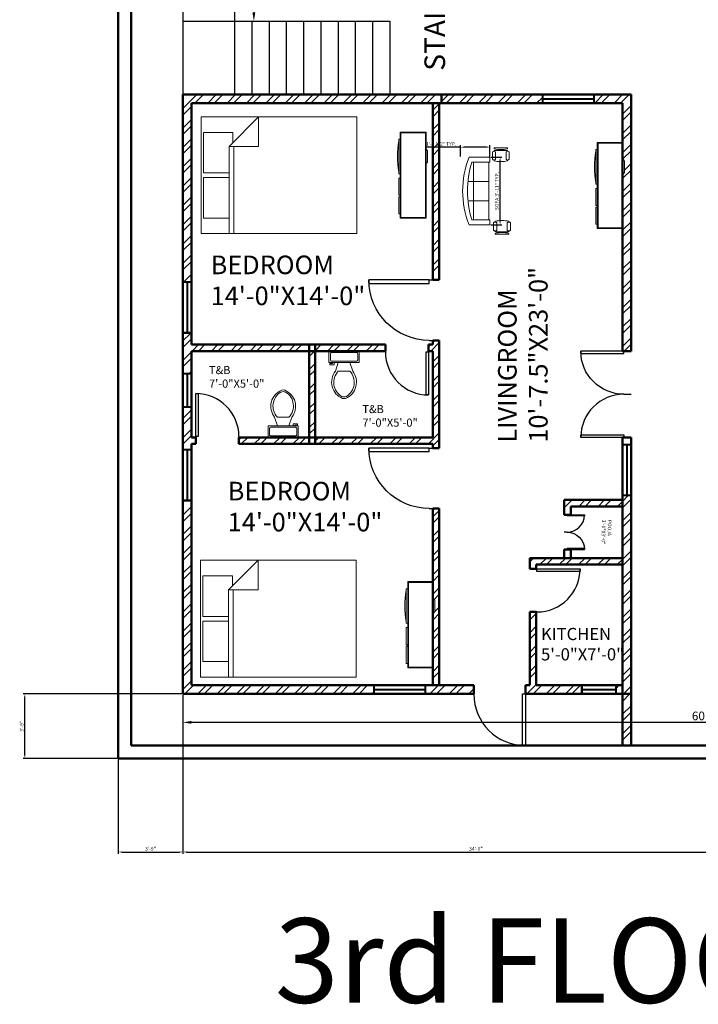
# Model space of a CAD drawing. Units: inches. Extents: x -12550 to 6516, y 1273 to 18700.
# Tile 12 of 19: x 4339 to 4811, y 1273 to 1958. Entities that reach past the tile are written whole.
import ezdxf

# ---------------------------------------------------------------- set-up
doc = ezdxf.new("R2010")
doc.units = ezdxf.units.IN
for name, color, linetype, lineweight in [('A-ANNO-DIMS', 2, 'Continuous', 18), ('A-ANNO-TEXT', 7, 'Continuous', 25), ('A-AREA-IDEN', 1, 'Continuous', 18), ('A-DOOR', 5, 'Continuous', 25), ('A-FLOR-STRS', 6, 'Continuous', 25), ('A-FURN', 8, 'Continuous', 18), ('A-GLAZ', 3, 'Continuous', 25), ('A-WALL', 7, 'Continuous', 50), ('A-WALL-PATT', 8, 'Continuous', 13)]:
    doc.layers.add(name, color=color, linetype=linetype, lineweight=lineweight)
doc.styles.get("Standard").update_dxf_attribs({"font": 'arial.ttf'})
doc.dimstyles.new('ISO-25', dxfattribs={"dimtxt": 2.5, "dimasz": 2.5, "dimexe": 1.25, "dimexo": 0.625, "dimtad": 1, "dimlunit": 4, "dimtxsty": 'Standard', "dimcen": 2.5, "dimadec": 0, "dimazin": 0, "dimtfac": 1, "dimtmove": 0, "dimatfit": 3, "dimfxl": 1, "dimarcsym": 0})
pattern_1 = [(45, (2434.941, 0), (-6.735192, 6.735192), []), (45, (2439.432, 0), (-6.735192, 6.735192), [])]

# ---------------------------------------------------------------- blocks, each defined once
blk = doc.blocks.new('*U2')
for p, q in [((0, 0), (0, -5)), ((30, 0), (30, -5))]:
    blk.add_line(p, q)
blk.add_lwpolyline([(0, 0), (0, 30), (1.75, 30), (1.75, 0)], close=True)
blk.add_arc((0, 0), 30, 0, 90)
blk = doc.blocks.new('Bed - Queen')
for p, q in [((0, -80.00003), (0, 0)), ((0, 0), (59.99999, 0)), ((59.99999, 0), (59.99999, -80.00003)), ((7.99999, -1.2), (28.79998, -1.2)), ((7.99999, -14.4), (7.99999, -1.2)), ((28.79998, -1.2), (28.79998, -14.4)), ((31.19999, -1.2), (51.99999, -1.2)), ((31.19999, -14.4), (31.19999, -1.2)), ((51.99999, -1.2), (51.99999, -16.4)), ((0, -14.4), (44.8, -14.4)), ((59.99999, -29.6), (44.8, -14.4)), ((44.8, -14.4), (44.8, -29.6)), ((44.8, -16.8), (0, -16.8)), ((51.99999, -16.4), (46.79936, -16.4)), ((44.8, -29.6), (59.99999, -29.6)), ((59.99999, -80.00003), (0, -80.00003))]:
    blk.add_line(p, q)
blk = doc.blocks.new('Toilet - top')
for p, q in [((9.5, -6), (9.5, -2)), ((-10, -8.5), (-8, -8.5)), ((-10, -9.5), (-10, -8.5)), ((-7, -9.5), (-10, -9.5)), ((-8, -8.5), (-8, -8)), ((-7, -8), (-7, -9.5)), ((-4, -8), (-6, -14)), ((4, -8), (6, -14)), ((4, -14), (-4, -14))]:
    blk.add_line(p, q)
blk.add_lwpolyline([(10.5, -8), (10.5, 0), (-10.5, 0), (-10.5, -8)], close=True)
for points in [[(-9.5, -2), (-9.5, -6)], [(8.5, -1), (-8.5, -1)], [(-8.5, -7), (8.5, -7)]]:
    blk.add_lwpolyline(points)
for centre, radius, start, end in [((-8.62, -1.88), 0.884, 81.8699, 188.1301), ((-8.62, -6.12), 0.884, 171.8699, 278.1301), ((8.62, -1.88), 0.884, 351.8699, 98.1301), ((8.62, -6.12), 0.884, 261.8699, 8.1301), ((3.52, -21.58), 12.17, 141.46911, 247.97143), ((4.2, -21.82), 11.33, 136.36773, 238.94682), ((-3.52, -21.58), 12.17, 292.02843, 38.53071), ((-4.2, -21.82), 11.33, 301.05301, 43.63209), ((0, -27.88), 4, 245.73182, 294.26817), ((0, -29), 4, 254.86053, 285.13947)]:
    blk.add_arc(centre, radius, start, end)
blk = doc.blocks.new('Entertainment Center')
for p, q in [((-4, 0), (-5, -1)), ((4, 0), (-4, 0)), ((5, -1), (4, 0)), ((-17, -19), (-17, -1)), ((-17, -1), (43, -1)), ((-16.5, -18.5), (-16.5, -1.5)), ((-16.5, -1.5), (42.5, -1.5)), ((42.5, -1.5), (42.5, -18.5)), ((43, -1), (43, -19)), ((43, -19), (-17, -19)), ((42.5, -18.5), (-16.5, -18.5)), ((-12, -20), (-12, -19)), ((12, -20), (-12, -20)), ((12, -19), (12, -20)), ((15, -20), (15, -19)), ((27, -20), (15, -20)), ((27, -19), (27, -20)), ((28, -20), (28, -19)), ((40, -20), (28, -20)), ((40, -19), (40, -20))]:
    blk.add_line(p, q)
blk.add_arc((0, 40), 61, 259.6111, 280.3889)
blk = doc.blocks.new('Sofa - Roundback 7 ft.')
for p, q in [((-36.000027, -34), (-36.000027, -11.4696)), ((-12.00002, -32.4421), (-12.00003, -6.5971)), ((11.99997, -32.4421), (11.99998, -6.5971)), ((35.99998, -34), (35.99998, -11.4696)), ((-35.999844, -13.3819), (35.9998, -13.3819)), ((-36.000027, -32.4421), (35.99998, -32.4421))]:
    blk.add_line(p, q)
for points in [[(-36.000027, -34), (-42.000027, -34), (-42.000027, -8)], [(41.99998, -8), (41.99998, -34), (35.99998, -34)]]:
    blk.add_lwpolyline(points)
for centre, radius, start, end in [((0, -114.25), 114.25, 68.43141, 111.5686), ((-0.00001, -127.1968), 121.1968, 72.72033, 107.2797)]:
    blk.add_arc(centre, radius, start, end)
blk = doc.blocks.new('Chair - Desk')
for p, q in [((-8.5, 0), (-8.5, -1)), ((-8.5, 0), (8.5, 0)), ((8.5, 0), (8.5, -1)), ((-10.5, -5), (-10.5, -14)), ((-8.5, -3), (-8.5, -4)), ((-8.5, -3), (8.5, -3)), ((-6.5, -14), (-6.5, -5)), ((-2, -3), (-2, -1.9355)), ((2, -1.9576), (2, -3)), ((6.5, -5), (6.5, -14)), ((8.5, -3), (8.5, -4)), ((10.5, -14), (10.5, -5)), ((-8.5, -15), (-8.5, -16)), ((8.5, -15), (8.5, -16))]:
    blk.add_line(p, q)
for centre, radius, start, end in [((-8.5, -6.5), 2.5, 36.8699, 143.1301), ((0, 34.625), 36.625, 256.5803, 283.4197), ((8.5, -6.5), 2.5, 36.8699, 143.1301), ((-8.5, -12.5), 2.5, 216.8699, 323.1301), ((0, 19.625), 36.625, 256.5803, 283.4197), ((8.5, -12.5), 2.5, 216.8699, 323.1301)]:
    blk.add_arc(centre, radius, start, end)
blk = doc.blocks.new('*D48')
at = {"layer": 'A-ANNO-DIMS', "color": 0, "lineweight": -2, "transparency": 16777216}
for p, q in [((4489.26, 2008.25), (4503.3, 2008.25)), ((4502.05, 2002.25), (4502.05, 1963.25)), ((4489.26, 1957.25), (4503.3, 1957.25))]:
    blk.add_line(p, q, dxfattribs=at)
at = {"layer": 'A-ANNO-DIMS', "color": 0, "transparency": 16777216}
for points in [[(4501.05, 2002.25), (4503.05, 2002.25), (4502.05, 2008.25)], [(4501.05, 1963.25), (4503.05, 1963.25), (4502.05, 1957.25)]]:
    blk.add_solid(points, dxfattribs=at)
at = {"layer": 'Defpoints', "color": 0, "transparency": 16777216}
for p in [(4488.63, 2008.25), (4488.63, 1957.25), (4502.05, 1957.25)]:
    blk.add_point(p, dxfattribs=at)
at = {"layer": 'A-ANNO-DIMS', "color": 0, "transparency": 16777216, "insert": (4498.36, 1982.75), "char_height": 6, "attachment_point": 5, "rotation": 90}
blk.add_mtext('4\'-3"', dxfattribs=at)
blk = doc.blocks.new('*D43')
at = {"layer": 'A-ANNO-DIMS', "color": 0, "lineweight": -2, "transparency": 16777216}
for p, q in [((4452.63, 1488.62), (4452.63, 1468.21)), ((5172.63, 1488.62), (5172.63, 1468.21)), ((5166.63, 1469.46), (4458.63, 1469.46))]:
    blk.add_line(p, q, dxfattribs=at)
at = {"layer": 'A-ANNO-DIMS', "color": 0, "transparency": 16777216}
for points in [[(4458.63, 1470.46), (4458.63, 1468.46), (4452.63, 1469.46)], [(5166.63, 1470.46), (5166.63, 1468.46), (5172.63, 1469.46)]]:
    blk.add_solid(points, dxfattribs=at)
at = {"layer": 'Defpoints', "color": 0, "transparency": 16777216}
for p in [(4452.63, 1489.25), (5172.63, 1489.25), (4452.63, 1469.46)]:
    blk.add_point(p, dxfattribs=at)
at = {"layer": 'A-ANNO-DIMS', "color": 0, "transparency": 16777216, "insert": (4812.63, 1473.15), "char_height": 6, "attachment_point": 5}
blk.add_mtext("60'", dxfattribs=at)
blk = doc.blocks.new('WIN-3FT')
for p, q in [((0, 0), (0, 6)), ((0, 6), (36.02, 6)), ((36.02, 0), (0, 0)), ((0.5, 0), (0.5, 6)), ((35.52, 3.2), (0.5, 3.2)), ((35.52, 2.8), (0.5, 2.8)), ((35.52, 6), (35.52, 0)), ((36.02, 6), (36.02, 0))]:
    blk.add_line(p, q)
blk = doc.blocks.new('WIN-2FT')
for p, q in [((0, 0), (0, 24.02)), ((0, 24.02), (6, 24.02)), ((0, 23.52), (6, 23.52)), ((2.8, 0.5), (2.8, 23.52)), ((3.2, 0.5), (3.2, 23.52)), ((6, 24.02), (6, 0)), ((6, 0.5), (0, 0.5)), ((6, 0), (0, 0))]:
    blk.add_line(p, q)
blk = doc.blocks.new('*D75')
at = {"layer": 'A-ANNO-DIMS', "color": 0, "lineweight": -2, "transparency": 16777216}
for p, q in [((4667.04, 1862.64), (4674.71, 1862.64)), ((4673.46, 1818.14), (4673.46, 1860.14)), ((4667.04, 1815.64), (4674.71, 1815.64))]:
    blk.add_line(p, q, dxfattribs=at)
at = {"layer": 'A-ANNO-DIMS', "color": 0, "transparency": 16777216}
for points in [[(4673.05, 1860.14), (4673.88, 1860.14), (4673.46, 1862.64)], [(4673.05, 1818.14), (4673.88, 1818.14), (4673.46, 1815.64)]]:
    blk.add_solid(points, dxfattribs=at)
at = {"layer": 'Defpoints', "color": 0, "transparency": 16777216}
for p in [(4666.41, 1862.64), (4673.46, 1862.64), (4666.41, 1815.64)]:
    blk.add_point(p, dxfattribs=at)
at = {"layer": 'A-ANNO-DIMS', "color": 0, "transparency": 16777216, "insert": (4671.54, 1839.14), "char_height": 2.5, "attachment_point": 5, "rotation": 90}
blk.add_mtext('SOFA 3\'-11" TYP.', dxfattribs=at)
blk = doc.blocks.new('*D76')
at = {"layer": 'A-ANNO-DIMS', "color": 0, "lineweight": -2, "transparency": 16777216}
for p, q in [((4645.9, 1863.26), (4645.9, 1870.94)), ((4666.41, 1863.26), (4666.41, 1870.94)), ((4645.9, 1869.69), (4621.32, 1869.69)), ((4663.91, 1869.69), (4648.4, 1869.69))]:
    blk.add_line(p, q, dxfattribs=at)
at = {"layer": 'A-ANNO-DIMS', "color": 0, "transparency": 16777216}
for points in [[(4648.4, 1870.1), (4648.4, 1869.27), (4645.9, 1869.69)], [(4663.91, 1870.1), (4663.91, 1869.27), (4666.41, 1869.69)]]:
    blk.add_solid(points, dxfattribs=at)
at = {"layer": 'Defpoints', "color": 0, "transparency": 16777216}
for p in [(4645.9, 1869.69), (4645.9, 1862.64), (4666.41, 1862.64)]:
    blk.add_point(p, dxfattribs=at)
at = {"layer": 'A-ANNO-DIMS', "color": 0, "transparency": 16777216, "insert": (4632.36, 1871.61), "char_height": 2.5, "attachment_point": 5}
blk.add_mtext('1\'-8 1/2" TYP.', dxfattribs=at)
blk = doc.blocks.new('*D114')
at = {"layer": 'A-ANNO-DIMS', "color": 0, "lineweight": -2, "transparency": 16777216}
for p, q in [((4452.63, 1488.62), (4452.63, 1378)), ((4407.63, 1443.62), (4407.63, 1378)), ((4410.13, 1379.25), (4450.13, 1379.25))]:
    blk.add_line(p, q, dxfattribs=at)
at = {"layer": 'A-ANNO-DIMS', "color": 0, "transparency": 16777216}
for points in [[(4410.13, 1379.66), (4410.13, 1378.83), (4407.63, 1379.25)], [(4450.13, 1379.66), (4450.13, 1378.83), (4452.63, 1379.25)]]:
    blk.add_solid(points, dxfattribs=at)
at = {"layer": 'Defpoints', "color": 0, "transparency": 16777216}
for p in [(4452.63, 1489.25), (4407.63, 1444.25), (4452.63, 1379.25)]:
    blk.add_point(p, dxfattribs=at)
at = {"layer": 'A-ANNO-DIMS', "color": 0, "transparency": 16777216, "insert": (4430.13, 1381.15), "char_height": 2.5, "attachment_point": 5}
blk.add_mtext('3\'-9"', dxfattribs=at)
blk = doc.blocks.new('*D115')
at = {"layer": 'A-ANNO-DIMS', "color": 0, "lineweight": -2, "transparency": 16777216}
for p, q in [((4452.63, 1488.62), (4452.63, 1378)), ((4860.63, 1488.62), (4860.63, 1378)), ((4455.13, 1379.25), (4858.13, 1379.25))]:
    blk.add_line(p, q, dxfattribs=at)
at = {"layer": 'A-ANNO-DIMS', "color": 0, "transparency": 16777216}
for points in [[(4455.13, 1379.66), (4455.13, 1378.83), (4452.63, 1379.25)], [(4858.13, 1379.66), (4858.13, 1378.83), (4860.63, 1379.25)]]:
    blk.add_solid(points, dxfattribs=at)
at = {"layer": 'Defpoints', "color": 0, "transparency": 16777216}
for p in [(4452.63, 1489.25), (4860.63, 1489.25), (4860.63, 1379.25)]:
    blk.add_point(p, dxfattribs=at)
at = {"layer": 'A-ANNO-DIMS', "color": 0, "transparency": 16777216, "insert": (4656.63, 1381.15), "char_height": 2.5, "attachment_point": 5}
blk.add_mtext('34\'-0"', dxfattribs=at)
blk = doc.blocks.new('*D119')
at = {"layer": 'A-ANNO-DIMS', "color": 0, "lineweight": -2, "transparency": 16777216}
for p, q in [((4452.01, 1489.25), (4341.38, 1489.25)), ((4342.63, 1446.75), (4342.63, 1486.75)), ((4407.01, 1444.25), (4341.38, 1444.25))]:
    blk.add_line(p, q, dxfattribs=at)
at = {"layer": 'A-ANNO-DIMS', "color": 0, "transparency": 16777216}
for points in [[(4342.21, 1486.75), (4343.05, 1486.75), (4342.63, 1489.25)], [(4342.21, 1446.75), (4343.05, 1446.75), (4342.63, 1444.25)]]:
    blk.add_solid(points, dxfattribs=at)
at = {"layer": 'Defpoints', "color": 0, "transparency": 16777216}
for p in [(4342.63, 1489.25), (4452.63, 1489.25), (4407.63, 1444.25)]:
    blk.add_point(p, dxfattribs=at)
at = {"layer": 'A-ANNO-DIMS', "color": 0, "transparency": 16777216, "insert": (4340.73, 1466.75), "char_height": 2.5, "attachment_point": 5, "rotation": 90}
blk.add_mtext('3\'-9"', dxfattribs=at)

msp = doc.modelspace()

# ---------------------------------------------------------------- hatches: boundary and pattern name
at = {"layer": 'A-WALL-PATT'}
h = msp.add_hatch(dxfattribs=at)
h.set_pattern_fill('ANSI32', color=256)
h.set_pattern_definition(pattern_1)
h.paths.add_polyline_path([(4458.63, 1900.247), (4632.63, 1900.247), (4632.63, 1906.247), (4452.63, 1906.247), (4452.63, 1776.138), (4458.63, 1776.138)])
h = msp.add_hatch(dxfattribs=at)
h.set_pattern_fill('ANSI32', color=256)
h.set_pattern_definition(pattern_1)
h.paths.add_polyline_path([(4702.882, 1906.247), (4632.63, 1906.247), (4632.63, 1900.247), (4702.882, 1900.247)])
h = msp.add_hatch(dxfattribs=at)
h.set_pattern_fill('ANSI32', color=256)
h.set_pattern_definition(pattern_1)
h.paths.add_polyline_path([(4764.63, 1906.247), (4738.899, 1906.247), (4738.899, 1900.247), (4758.63, 1900.247), (4758.63, 1872.972), (4759.13, 1872.972), (4759.13, 1860.972), (4760.13, 1859.972), (4760.13, 1851.972), (4759.13, 1850.972), (4759.13, 1812.972), (4758.63, 1727.747), (4759.63, 1727.747), (4764.63, 1727.747)])
h = msp.add_hatch(dxfattribs=at)
h.set_pattern_fill('ANSI32', color=256)
h.set_pattern_definition(pattern_1)
h.paths.add_polyline_path([(4631.13, 1900.247), (4626.63, 1900.247), (4626.63, 1777.247), (4631.13, 1777.247)], flags=17)
h = msp.add_hatch(dxfattribs=at)
h.set_pattern_fill('ANSI32', color=256)
h.set_pattern_definition(pattern_1)
h.paths.add_polyline_path([(4540.63, 1732.247), (4458.63, 1732.247), (4458.63, 1740.121), (4452.63, 1740.121), (4452.63, 1712.466), (4458.63, 1712.466), (4458.63, 1727.747), (4540.63, 1727.747)])
h = msp.add_hatch(dxfattribs=at)
h.set_pattern_fill('ANSI32', color=256)
h.set_pattern_definition(pattern_1)
h.paths.add_polyline_path([(4631.13, 1735.247), (4626.63, 1735.247), (4626.63, 1732.247), (4623.63, 1732.247), (4623.63, 1727.747), (4626.63, 1727.747), (4626.63, 1667.747), (4544.63, 1667.747), (4544.63, 1663.247), (4626.63, 1663.247), (4626.63, 1660.247), (4631.13, 1660.247)])
h = msp.add_hatch(dxfattribs=at)
h.set_pattern_fill('ANSI32', color=256)
h.set_pattern_definition(pattern_1)
h.paths.add_polyline_path([(4544.63, 1727.747), (4540.63, 1727.747), (4540.63, 1667.747), (4544.63, 1667.747)])
h = msp.add_hatch(dxfattribs=at)
h.set_pattern_fill('ANSI32', color=256)
h.set_pattern_definition(pattern_1)
h.paths.add_polyline_path([(4593.63, 1732.247), (4544.63, 1732.247), (4544.63, 1727.747), (4593.63, 1727.747)], flags=17)
h = msp.add_hatch(dxfattribs=at)
h.set_pattern_fill('ANSI32', color=256)
h.set_pattern_definition(pattern_1)
h.paths.add_polyline_path([(4458.63, 1688.449), (4452.63, 1688.449), (4452.63, 1659.453), (4458.63, 1659.453), (4458.63, 1663.247), (4461.63, 1663.247), (4461.63, 1667.747), (4458.63, 1667.747)])
h = msp.add_hatch(dxfattribs=at)
h.set_pattern_fill('ANSI32', color=256)
h.set_pattern_definition(pattern_1)
h.paths.add_polyline_path([(4540.63, 1667.747), (4491.63, 1667.747), (4491.63, 1663.247), (4540.63, 1663.247)])
h = msp.add_hatch(dxfattribs=at)
h.set_pattern_fill('ANSI32', color=256)
h.set_pattern_definition(pattern_1)
h.paths.add_polyline_path([(4758.63, 1624.247), (4718.13, 1624.247), (4718.13, 1613.747), (4720.13, 1613.747), (4722.63, 1613.747), (4722.63, 1619.747), (4758.63, 1619.747)])
h = msp.add_hatch(dxfattribs=at)
h.set_pattern_fill('ANSI32', color=256)
h.set_pattern_definition(pattern_1)
h.paths.add_polyline_path([(4764.63, 1627.032), (4758.63, 1627.032), (4758.63, 1495.247), (4754.235, 1495.247), (4754.235, 1489.247), (4764.63, 1489.247)])
h = msp.add_hatch(dxfattribs=at)
h.set_pattern_fill('ANSI32', color=256)
h.set_pattern_definition(pattern_1)
h.paths.add_polyline_path([(4458.63, 1623.435), (4452.63, 1623.435), (4452.63, 1489.247), (4585.581, 1489.247), (4585.581, 1495.247), (4458.63, 1495.247)])
h = msp.add_hatch(dxfattribs=at)
h.set_pattern_fill('ANSI32', color=256)
h.set_pattern_definition(pattern_1)
h.paths.add_polyline_path([(4631.13, 1618.247), (4626.63, 1618.247), (4626.63, 1567.365), (4627.13, 1567.365), (4627.13, 1555.365), (4628.13, 1554.365), (4628.13, 1546.365), (4627.13, 1545.365), (4627.13, 1507.365), (4626.63, 1495.247), (4631.13, 1495.247)])
h = msp.add_hatch(dxfattribs=at)
h.set_pattern_fill('ANSI32', color=256)
h.set_pattern_definition(pattern_1)
h.paths.add_polyline_path([(4758.63, 1583.747), (4694.13, 1583.747), (4694.13, 1576.247), (4698.63, 1576.247), (4698.63, 1579.247), (4758.63, 1579.247)])
h = msp.add_hatch(dxfattribs=at)
h.set_pattern_fill('ANSI32', color=256)
h.set_pattern_definition(pattern_1)
h.paths.add_polyline_path([(4730.218, 1495.247), (4698.63, 1495.247), (4698.63, 1546.247), (4694.13, 1546.247), (4694.13, 1495.247), (4691.13, 1495.247), (4691.13, 1489.247), (4730.218, 1489.247)])
h = msp.add_hatch(dxfattribs=at)
h.set_pattern_fill('ANSI32', color=256)
h.set_pattern_definition(pattern_1)
h.paths.add_polyline_path([(4655.13, 1495.247), (4621.598, 1495.247), (4621.598, 1489.247), (4655.13, 1489.247)])
h = msp.add_hatch(dxfattribs=at)
h.set_pattern_fill('ANSI32', color=256)
h.set_pattern_definition(pattern_1)
h.paths.add_polyline_path([(4764.63, 1489.247), (4758.63, 1489.247), (4758.63, 1453.247), (4764.63, 1453.247)])

# ---------------------------------------------------------------- linework, layer by layer
at = {"layer": 'A-FLOR-STRS'}
for p, q in [((4452.63, 2056.247), (4452.63, 1906.247)), ((4488.63, 2056.247), (4488.63, 1906.247)), ((4452.63, 1957.247), (4596.63, 1957.247)), ((4500.63, 1957.247), (4500.63, 1906.247)), ((4512.63, 1957.247), (4512.63, 1906.247)), ((4524.63, 1957.247), (4524.63, 1906.247)), ((4536.63, 1957.247), (4536.63, 1906.247)), ((4548.63, 1957.247), (4548.63, 1906.247)), ((4560.63, 1957.247), (4560.63, 1906.247)), ((4572.63, 1957.247), (4572.63, 1906.247)), ((4584.63, 1957.247), (4584.63, 1906.247)), ((4596.63, 1957.247), (4596.63, 1906.247)), ((4452.63, 1906.247), (4632.63, 1906.247))]:
    msp.add_line(p, q, dxfattribs=at)
at = {"layer": 'A-WALL'}
for p, q in [((4407.63, 1444.247), (4407.63, 2518.247)), ((4416.63, 1453.247), (4416.63, 2509.247)), ((4764.63, 1906.247), (4452.63, 1906.247)), ((4452.63, 1489.247), (4452.63, 1906.247)), ((4632.63, 1900.247), (4632.63, 1906.247)), ((4764.63, 1727.747), (4764.63, 1906.247)), ((4758.63, 1900.247), (4458.63, 1900.247)), ((4458.63, 1732.247), (4458.63, 1900.247)), ((4626.63, 1777.247), (4626.63, 1900.247)), ((4631.13, 1777.247), (4631.13, 1900.247)), ((4758.63, 1727.747), (4758.63, 1900.247)), ((4631.13, 1777.247), (4626.63, 1777.247)), ((4626.63, 1732.247), (4626.63, 1735.247)), ((4626.63, 1732.247), (4626.63, 1735.247)), ((4626.63, 1735.247), (4631.13, 1735.247)), ((4631.13, 1660.247), (4631.13, 1735.247)), ((4593.63, 1732.247), (4458.63, 1732.247)), ((4593.63, 1727.747), (4458.63, 1727.747)), ((4458.63, 1667.747), (4458.63, 1727.747)), ((4540.63, 1663.247), (4540.63, 1732.247)), ((4544.63, 1663.247), (4544.63, 1732.247)), ((4593.63, 1727.747), (4593.63, 1732.247)), ((4626.63, 1732.247), (4623.63, 1732.247)), ((4626.63, 1732.247), (4623.63, 1732.247)), ((4623.63, 1732.247), (4623.63, 1727.747)), ((4626.63, 1727.747), (4623.63, 1727.747)), ((4626.63, 1667.747), (4626.63, 1727.747)), ((4764.63, 1727.747), (4758.63, 1727.747)), ((4461.63, 1667.747), (4458.63, 1667.747)), ((4461.63, 1663.247), (4461.63, 1667.747)), ((4626.63, 1667.747), (4491.63, 1667.747)), ((4491.63, 1667.747), (4626.63, 1667.747)), ((4491.63, 1667.747), (4491.63, 1663.247)), ((4764.63, 1667.747), (4758.63, 1667.747)), ((4758.63, 1453.247), (4758.63, 1667.747)), ((4764.63, 1489.247), (4764.63, 1667.747)), ((4461.63, 1663.247), (4458.63, 1663.247)), ((4458.63, 1495.247), (4458.63, 1663.247)), ((4458.63, 1663.247), (4461.63, 1663.247)), ((4626.63, 1663.247), (4491.63, 1663.247)), ((4626.63, 1660.247), (4626.63, 1663.247)), ((4631.13, 1660.247), (4626.63, 1660.247)), ((4631.13, 1663.247), (4631.13, 1660.247)), ((4758.63, 1624.247), (4718.13, 1624.247)), ((4718.13, 1613.747), (4718.13, 1624.247)), ((4626.63, 1495.247), (4626.63, 1618.247)), ((4626.63, 1618.247), (4631.13, 1618.247)), ((4631.13, 1495.247), (4631.13, 1618.247)), ((4758.63, 1619.747), (4722.63, 1619.747)), ((4722.63, 1613.747), (4722.63, 1619.747)), ((4718.13, 1613.747), (4722.63, 1613.747)), ((4718.13, 1583.747), (4718.13, 1589.747)), ((4722.63, 1589.747), (4718.13, 1589.747)), ((4722.63, 1583.747), (4722.63, 1589.747)), ((4722.63, 1583.747), (4722.63, 1589.747)), ((4758.63, 1583.747), (4694.13, 1583.747)), ((4694.13, 1576.247), (4694.13, 1583.747)), ((4718.13, 1583.747), (4718.13, 1588.747)), ((4698.63, 1576.247), (4694.13, 1576.247)), ((4758.63, 1579.247), (4698.63, 1579.247)), ((4698.63, 1576.247), (4698.63, 1579.247)), ((4698.63, 1579.247), (4698.63, 1576.247)), ((4694.13, 1495.247), (4694.13, 1546.247)), ((4694.13, 1546.247), (4698.63, 1546.247)), ((4698.63, 1495.247), (4698.63, 1546.247)), ((4655.13, 1495.247), (4458.63, 1495.247)), ((4655.13, 1495.247), (4631.13, 1495.247)), ((4655.13, 1489.247), (4655.13, 1495.247)), ((4694.13, 1495.247), (4691.13, 1495.247)), ((4694.13, 1495.247), (4691.13, 1495.247)), ((4691.13, 1495.247), (4691.13, 1489.247)), ((4758.63, 1495.247), (4698.63, 1495.247)), ((4655.13, 1489.247), (4452.63, 1489.247)), ((4764.63, 1489.247), (4691.13, 1489.247)), ((4764.63, 1489.247), (4764.63, 1453.247)), ((4416.63, 1453.247), (5208.63, 1453.247)), ((4955.13, 1453.247), (4691.13, 1453.247)), ((4407.63, 1444.247), (5217.63, 1444.247))]:
    msp.add_line(p, q, dxfattribs=at)

# ---------------------------------------------------------------- block references
at = {"layer": 'A-DOOR'}
for p, xscale, yscale, zscale, rotation in [((4624.13, 1777.247), -1.4, 1.4, 1.4, 90), ((4624.13, 1660.247), -1.4, 1.4, 1.4, 90), ((4720.13, 1613.747), 0.399999999999997, 0.399999999999997, 0.399999999999997, 270), ((4720.13, 1589.747), -0.399999999999997, 0.399999999999997, 0.399999999999997, 270), ((4691.13, 1489.247), 1.199999999999999, 1.199999999999999, 1.199999999999999, 180)]:
    msp.add_blockref('*U2', p, dxfattribs=dict(at, xscale=xscale, yscale=yscale, zscale=zscale, rotation=rotation))
for p, rotation in [((4623.63, 1727.247), 180), ((4759.63, 1667.747), 90), ((4699.13, 1576.247), 270)]:
    msp.add_blockref('*U2', p, dxfattribs=dict(at, rotation=rotation))
at = {"layer": 'A-DOOR', "xscale": -1, "rotation": 90}
msp.add_blockref('*U2', (4759.63, 1727.747), dxfattribs=at)
at = {"layer": 'A-DOOR'}
msp.add_blockref('*U2', (4461.63, 1668.247), dxfattribs=at)
at = {"layer": 'A-FURN'}
for name, p, xscale, yscale, zscale, rotation in [('Bed - Queen', (4465.28, 1809.493), 1.354827908062564, 1.354827908062564, 1.354827908062564, 90), ('Sofa - Roundback 7 ft.', (4647.389, 1839.138), 0.5595223685495907, 0.5595223685495907, 0.5595223685495907, 90), ('Chair - Desk', (4674.829, 1809.138), 0.5595223685495907, 0.5595223685495907, 0.5595223685495907, 180), ('Bed - Queen', (4464.979, 1500.915), 1.354827908062564, 1.354827908062564, 1.354827908062564, 90)]:
    msp.add_blockref(name, p, dxfattribs=dict(at, xscale=xscale, yscale=yscale, zscale=zscale, rotation=rotation))
for name, p, rotation in [('Entertainment Center', (4622.971, 1863.204), 270), ('Entertainment Center', (4760.13, 1855.972), 270), ('Toilet - top', (4522.477, 1667.747), 180), ('Entertainment Center', (4628.13, 1550.365), 270)]:
    msp.add_blockref(name, p, dxfattribs=dict(at, rotation=rotation))
at = {"layer": 'A-FURN', "xscale": 0.5595223685495907, "yscale": 0.5595223685495907, "zscale": 0.5595223685495907}
msp.add_blockref('Chair - Desk', (4673.975, 1869.122), dxfattribs=at)
at = {"layer": 'A-FURN'}
msp.add_blockref('Toilet - top', (4564.841, 1727.747), dxfattribs=at)
at = {"layer": 'A-GLAZ'}
for name, p, rotation in [('WIN-3FT', (4738.899, 1906.247), 180), ('WIN-3FT', (4458.63, 1740.121), 90.00000000000175), ('WIN-2FT', (4458.63, 1712.467), 180), ('WIN-3FT', (4458.63, 1623.436), 90.00000000000163), ('WIN-3FT', (4764.63, 1627.032), 89.99999999999638), ('WIN-3FT', (4621.598, 1495.247), 180), ('WIN-2FT', (4730.218, 1495.247), 269.9999999999954)]:
    msp.add_blockref(name, p, dxfattribs=dict(at, rotation=rotation))

# ---------------------------------------------------------------- texts
at = {"layer": 'A-ANNO-TEXT', "insert": (4516.607, 1333.138), "char_height": 58.816, "attachment_point": 1}
msp.add_mtext('3rd FLOOR', dxfattribs=at)
at = {"layer": 'A-AREA-IDEN', "attachment_point": 1}
for s, width, gutter_width, insert, char_height, rotation in [('STAIRCASE', 2.19144, 71.795, (4620.807, 1922.837), 14.3589, 90), ('POOJA\\P3\'-0"X3\'-0"', 0.78585, 12.5, (4751.006, 1610.304), 2.5, 269.183853)]:
    msp.add_mtext_dynamic_manual_height_columns(s, width=width, gutter_width=gutter_width, heights=[0], dxfattribs=dict(at, insert=insert, char_height=char_height, rotation=rotation))
at = {"layer": 'A-AREA-IDEN', "char_height": 12.93169, "attachment_point": 1}
for insert in [(4471.967, 1794.217), (4483.848, 1636.812)]:
    msp.add_mtext('BEDROOM\\P14\'-0"X14\'-0"', dxfattribs=dict(at, insert=insert))
at = {"layer": 'A-AREA-IDEN', "insert": (4672.036, 1664.034), "char_height": 12.93169, "attachment_point": 1, "rotation": 90}
msp.add_mtext('LIVINGROOM\\P10\'-7.5"X23\'-0"', dxfattribs=at)
at = {"layer": 'A-AREA-IDEN', "attachment_point": 1}
for s, width, gutter_width, insert, char_height in [('T&B\\P7\'-0"X5\'-0"', 4.19569, 28.328, (4470.806, 1717.416), 5.66556), ('T&B\\P7\'-0"X5\'-0"', 4.19569, 28.328, (4577.568, 1690.282), 5.66556), ('KITCHEN\\P5\'-0"X7\'-0"', 1.29487, 42.422, (4701.952, 1535.176), 8.48435)]:
    msp.add_mtext_dynamic_manual_height_columns(s, width=width, gutter_width=gutter_width, heights=[0], dxfattribs=dict(at, insert=insert, char_height=char_height))

# ---------------------------------------------------------------- dimensions: what is measured, and where the dimension line sits
at = {"layer": 'A-ANNO-DIMS'}
for base, p1, p2, override, picture, middle in [((4502.052, 1957.247), (4488.63, 2008.247), (4488.63, 1957.247), {"dimtxt": 6, "dimasz": 6, "dimclrd": 0, "dimclre": 0, "dimclrt": 0}, '*D48', (4498.362, 1982.747)), ((4342.63, 1489.247), (4407.63, 1444.247), (4452.63, 1489.247), {"dimdec": 1, "dimlfac": 1, "dimrnd": 0, "dimzin": 1, "dimdsep": 46, "dimlunit": 4, "dimfrac": 2}, '*D119', (4340.728, 1466.747))]:
    dim = msp.add_linear_dim(base=base, p1=p1, p2=p2, angle=90, dimstyle='ISO-25', override=override, dxfattribs=at)
    dim.commit()
    dim.dimension.update_dxf_attribs({"geometry": picture, "text_midpoint": middle})
for base, p1, p2, angle, text, picture, middle in [((4645.897, 1869.688), (4666.413, 1862.638), (4645.897, 1862.638), 180, '<> TYP.', '*D76', (4632.358, 1871.606)), ((4673.463, 1862.638), (4666.413, 1815.638), (4666.413, 1862.638), 90, 'SOFA <> TYP.', '*D75', (4671.544, 1839.138))]:
    dim = msp.add_linear_dim(base=base, p1=p1, p2=p2, angle=angle, text=text, dimstyle='ISO-25', override={"dimdec": 1, "dimrnd": 0, "dimzin": 1, "dimlunit": 4, "dimfrac": 2}, dxfattribs=at)
    dim.commit()
    dim.dimension.update_dxf_attribs({"geometry": picture, "text_midpoint": middle})
for base, p1, p2, override, picture, middle in [((4452.63, 1379.247), (4407.63, 1444.247), (4452.63, 1489.247), {"dimdec": 1, "dimlfac": 1, "dimrnd": 0, "dimzin": 1, "dimdsep": 46, "dimlunit": 4, "dimfrac": 2}, '*D114', (4430.13, 1381.15)), ((4452.63, 1469.461), (5172.63, 1489.247), (4452.63, 1489.247), {"dimtxt": 6, "dimasz": 6, "dimclrd": 0, "dimclre": 0, "dimclrt": 0}, '*D43', (4812.63, 1473.15)), ((4860.63, 1379.247), (4452.63, 1489.247), (4860.63, 1489.247), {"dimdec": 1, "dimlfac": 1, "dimrnd": 0, "dimzin": 1, "dimdsep": 46, "dimlunit": 4, "dimfrac": 2}, '*D115', (4656.63, 1381.15))]:
    dim = msp.add_linear_dim(base=base, p1=p1, p2=p2, dimstyle='ISO-25', override=override, dxfattribs=at)
    dim.commit()
    dim.dimension.update_dxf_attribs({"geometry": picture, "text_midpoint": middle})

doc.saveas('drawing.dxf')
